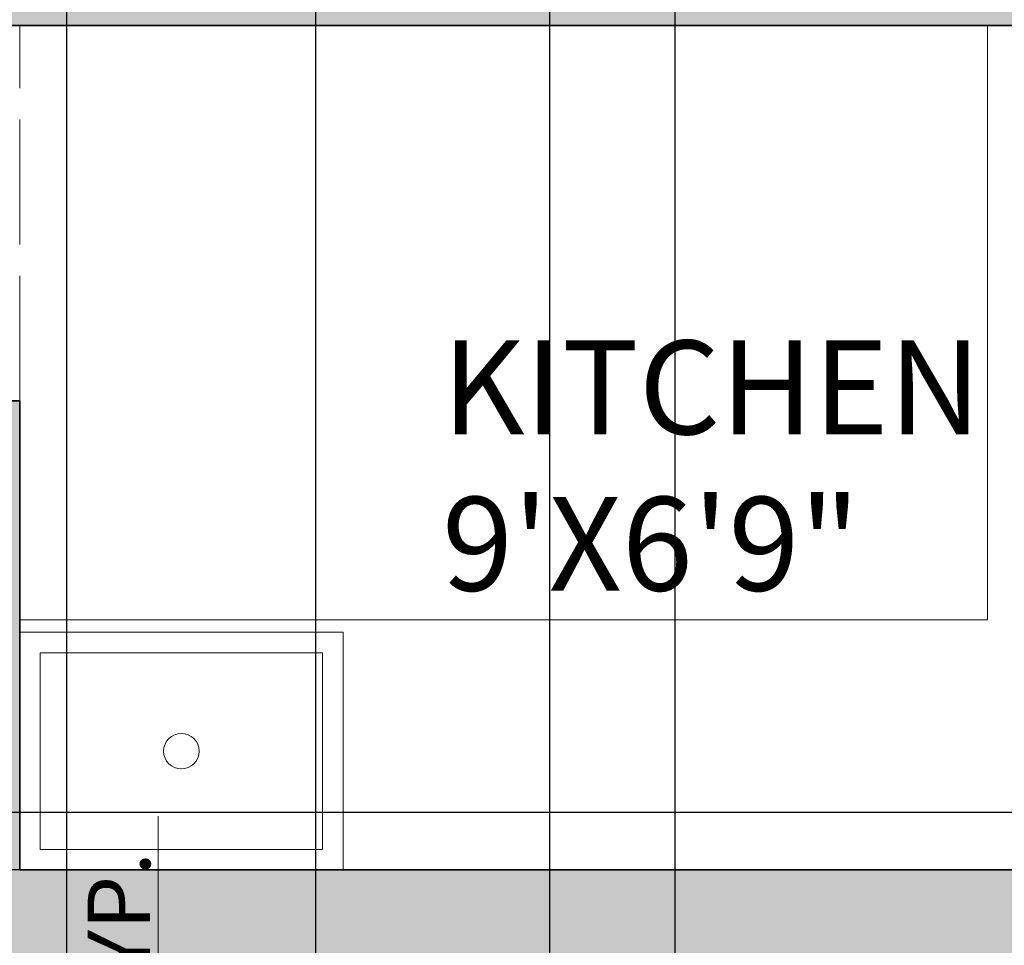
# Model space of a CAD drawing. Units: inches. Extents: x 2696 to 3240, y 1564 to 2310.
# Tile 65 of 76: x 3074 to 3168, y 1982 to 2071. Entities that reach past the tile are written whole.
import ezdxf

# ---------------------------------------------------------------- set-up
doc = ezdxf.new("R2010")
doc.units = ezdxf.units.IN
doc.linetypes.add('ACAD_ISO02W100', pattern=[15, 12, -3])
for name, color, linetype, lineweight in [('A-ANNO-DIMS', 3, 'Continuous', 18), ('A-AREA-IDEN', 7, 'Continuous', 18), ('A-FLOR-CASE', 8, 'Continuous', 18), ('A-FLOR-FIXT', 8, 'Continuous', 18), ('A-WALL', 7, 'Continuous', 35), ('A-WALL-OVHD', 7, 'ACAD_ISO02W100', 18), ('A-WALL-PATT', 9, 'Continuous', 13)]:
    doc.layers.add(name, color=color, linetype=linetype, lineweight=lineweight)
doc.styles.add('TIMES NEW', font='times.ttf')
doc.styles.add('YQ_DIM', font='SUPEROS.SHX', dxfattribs={"width": 0.8, "bigfont": 'HZDX.SHX'})
doc.dimstyles.new('Siddhuu', dxfattribs={"dimtxt": 6, "dimasz": 2.5, "dimexe": 1.25, "dimexo": 0.625, "dimtad": 1, "dimdec": 1, "dimlunit": 4, "dimtxsty": 'TIMES NEW', "dimcen": 2.5, "dimclrd": 256, "dimclre": 1, "dimclrt": 7, "dimadec": 0, "dimazin": 0, "dimtfac": 1, "dimtdec": 1, "dimtmove": 0, "dimatfit": 3, "dimfxl": 1, "dimtolj": 1, "dimlwd": -1, "dimarcsym": 0})

# ---------------------------------------------------------------- blocks, each defined once
blk = doc.blocks.new('SINK-KITCHEN')
for points in [[(0, 22.797), (31.038, 22.797), (31.038, 0), (0, 0)], [(1.972, 20.824), (29.066, 20.824), (29.066, 1.972), (1.972, 1.972)]]:
    blk.add_lwpolyline(points, close=True)
blk.add_circle((15.519, 11.398), 1.705)
blk = doc.blocks.new('*D48')
at = {"layer": 'A-ANNO-DIMS', "transparency": 16777216}
for p, q in [((3087, 1884.201), (3087, 1994.355)), ((3087, 1827.443), (3087, 1881.701))]:
    blk.add_line(p, q, dxfattribs=at)
at = {"layer": 'A-ANNO-DIMS', "color": 1, "lineweight": -2, "transparency": 16777216}
for p, q in [((3078.736, 1884.201), (3088.25, 1884.201)), ((3078.736, 1824.943), (3088.25, 1824.943))]:
    blk.add_line(p, q, dxfattribs=at)
at = {"layer": 'A-ANNO-DIMS', "transparency": 16777216}
for points in [[(3086.583, 1881.701), (3087.417, 1881.701), (3087, 1884.201)], [(3086.583, 1827.443), (3087.417, 1827.443), (3087, 1824.943)]]:
    blk.add_solid(points, dxfattribs=at)
at = {"layer": 'Defpoints', "color": 0, "transparency": 16777216}
for p in [(3078.111, 1884.201), (3087, 1884.201), (3078.111, 1824.943)]:
    blk.add_point(p, dxfattribs=at)
at = {"layer": 'A-ANNO-DIMS', "color": 7, "transparency": 16777216, "insert": (3083.232, 1940.528), "char_height": 6, "attachment_point": 5, "rotation": 90, "style": 'TIMES NEW'}
blk.add_mtext('\\A1;SECTIONAL 4\'-11 1/2" TYP.', dxfattribs=at)
blk = doc.blocks.new('*D54')
at = {"layer": 'A-ANNO-DIMS', "color": 1, "lineweight": -2, "transparency": 16777216}
for p, q in [((3124.611, 1893.826), (3124.611, 2298.451)), ((3136.611, 1893.826), (3136.611, 2298.451))]:
    blk.add_line(p, q, dxfattribs=at)
at = {"layer": 'A-ANNO-DIMS', "transparency": 16777216}
for p, q in [((3127.111, 2297.201), (3134.111, 2297.201)), ((3136.611, 2297.201), (3155.757, 2297.201))]:
    blk.add_line(p, q, dxfattribs=at)
for points in [[(3127.111, 2297.618), (3127.111, 2296.784), (3124.611, 2297.201)], [(3134.111, 2297.618), (3134.111, 2296.784), (3136.611, 2297.201)]]:
    blk.add_solid(points, dxfattribs=at)
at = {"layer": 'Defpoints', "color": 0, "transparency": 16777216}
for p in [(3136.611, 2297.201), (3124.611, 1893.201), (3136.611, 1893.201)]:
    blk.add_point(p, dxfattribs=at)
at = {"layer": 'A-ANNO-DIMS', "color": 7, "transparency": 16777216, "insert": (3147.434, 2300.878), "char_height": 6, "attachment_point": 5, "style": 'TIMES NEW'}
blk.add_mtext('\\A1;1\'-0"', dxfattribs=at)
blk = doc.blocks.new('*D65')
at = {"layer": 'A-ANNO-DIMS', "color": 1, "lineweight": -2, "transparency": 16777216}
for p, q in [((3078.209, 2122.076), (3078.209, 1568.951)), ((3102.111, 2122.076), (3102.111, 1568.951))]:
    blk.add_line(p, q, dxfattribs=at)
at = {"layer": 'A-ANNO-DIMS', "transparency": 16777216}
blk.add_line((3080.709, 1570.201), (3099.611, 1570.201), dxfattribs=at)
for points in [[(3080.709, 1570.618), (3080.709, 1569.784), (3078.209, 1570.201)], [(3099.611, 1570.618), (3099.611, 1569.784), (3102.111, 1570.201)]]:
    blk.add_solid(points, dxfattribs=at)
at = {"layer": 'Defpoints', "color": 0, "transparency": 16777216}
for p in [(3078.209, 2122.701), (3102.111, 2122.701), (3102.111, 1570.201)]:
    blk.add_point(p, dxfattribs=at)
at = {"layer": 'A-ANNO-DIMS', "color": 7, "transparency": 16777216, "insert": (3090.16, 1573.878), "char_height": 6, "attachment_point": 5, "style": 'TIMES NEW'}
blk.add_mtext('\\A1;2\'-0"', dxfattribs=at)
blk = doc.blocks.new('*D77')
at = {"layer": 'A-ANNO-DIMS', "transparency": 16777216}
for p, q in [((2710.611, 1997.201), (2710.611, 2030.601)), ((2710.611, 1989.201), (2710.611, 1994.701)), ((2710.611, 1986.701), (2710.611, 1984.201))]:
    blk.add_line(p, q, dxfattribs=at)
at = {"layer": 'A-ANNO-DIMS', "color": 1, "lineweight": -2, "transparency": 16777216}
for p, q in [((3189.986, 1994.701), (2709.361, 1994.701)), ((3189.986, 1989.201), (2709.361, 1989.201))]:
    blk.add_line(p, q, dxfattribs=at)
at = {"layer": 'A-ANNO-DIMS', "transparency": 16777216}
for points in [[(2710.195, 1997.201), (2711.028, 1997.201), (2710.611, 1994.701)], [(2710.195, 1986.701), (2711.028, 1986.701), (2710.611, 1989.201)]]:
    blk.add_solid(points, dxfattribs=at)
at = {"layer": 'Defpoints', "color": 0, "transparency": 16777216}
for p in [(2710.611, 1994.701), (3190.611, 1994.701), (3190.611, 1989.201)]:
    blk.add_point(p, dxfattribs=at)
at = {"layer": 'A-ANNO-DIMS', "color": 7, "transparency": 16777216, "insert": (2706.85, 2015.151), "char_height": 6, "attachment_point": 5, "rotation": 90, "style": 'TIMES NEW'}
blk.add_mtext('\\A1;0\'-5 1/2"', dxfattribs=at)

msp = doc.modelspace()

# ---------------------------------------------------------------- hatches: boundary and pattern name
at = {"layer": 'A-WALL-PATT', "transparency": 33554556}
h = msp.add_hatch(color=256, dxfattribs=at)
h.dxf.hatch_style = 1
h.paths.add_polyline_path([(2879.111, 2253.201), (2905.91, 2253.201), (2905.91, 2262.201), (2841.889, 2262.201), (2841.889, 2253.201), (2870.111, 2253.201), (2870.111, 2176.601), (2965.709, 2176.601), (2965.709, 2206.701), (2973.583, 2206.701), (2973.583, 2215.701), (2965.709, 2215.701), (2965.709, 2262.201), (2929.91, 2262.201), (2929.91, 2253.201), (2956.709, 2253.201), (2956.709, 2185.601), (2879.111, 2185.601)])
h.paths.add_polyline_path([(2782.834, 2262.201), (2745.611, 2262.201), (2745.611, 2228.729), (2754.611, 2228.729), (2754.611, 2253.201), (2782.834, 2253.201)])
h.paths.add_polyline_path([(2754.611, 2136.201), (2965.709, 2136.201), (2965.709, 2145.201), (2879.111, 2145.201), (2879.111, 2147.074), (2877.34, 2147.074), (2870.111, 2147.074), (2870.111, 2145.201), (2754.611, 2145.201), (2754.611, 2169.674), (2745.611, 2169.674), (2745.611, 2000.201), (2754.611, 2000.201), (2754.611, 2019.201), (2849.083, 2019.201), (2849.083, 2023.701), (2841.209, 2023.701), (2841.209, 2051.827), (2836.709, 2051.827), (2836.709, 2023.701), (2754.611, 2023.701), (2754.611, 2091.201), (2836.709, 2091.201), (2836.709, 2087.827), (2841.209, 2087.827), (2841.209, 2095.701), (2754.611, 2095.701)])
h.paths.add_polyline_path([(2965.709, 2136.201), (2956.709, 2136.201), (2956.709, 2023.701), (2885.083, 2023.701), (2885.083, 2019.201), (2956.709, 2019.201), (2956.709, 1950.575), (2965.709, 1950.575), (2965.709, 1980.201), (2973.583, 1980.201), (2973.583, 1989.201), (2965.709, 1989.201)])
h.paths.add_polyline_path([(2754.611, 1906.701), (2880.209, 1906.701), (2884.709, 1906.701), (2956.709, 1906.701), (2956.709, 1792.701), (2944.709, 1792.701), (2944.709, 1783.701), (2956.709, 1783.701), (2956.709, 1740.201), (2884.709, 1740.201), (2884.709, 1783.701), (2896.709, 1783.701), (2896.709, 1792.701), (2884.709, 1792.701), (2884.709, 1846.701), (2880.209, 1846.701), (2880.209, 1740.201), (2754.611, 1740.201), (2754.611, 1777.201), (2745.611, 1777.201), (2745.611, 1692.701), (2754.611, 1692.701), (2754.611, 1731.201), (2956.709, 1731.201), (2956.709, 1723.327), (2965.709, 1723.327), (2965.709, 1884.201), (2973.583, 1884.201), (2973.583, 1893.201), (2965.709, 1893.201), (2965.709, 1914.575), (2956.709, 1914.575), (2956.709, 1911.201), (2754.611, 1911.201), (2754.611, 1930.201), (2745.611, 1930.201), (2745.611, 1817.201), (2754.611, 1817.201), (2754.611, 1854.201), (2826.611, 1854.201), (2826.611, 1868.827), (2822.111, 1868.827), (2822.111, 1858.701), (2754.611, 1858.701)])
h.paths.add_polyline_path([(2965.709, 1656.201), (3008.237, 1656.201), (3008.237, 1665.201), (2965.709, 1665.201), (2965.709, 1693.327), (2956.709, 1693.327), (2956.709, 1686.201), (2934.583, 1686.201), (2934.583, 1681.701), (2956.709, 1681.701), (2956.709, 1614.201), (2896.709, 1614.201), (2896.709, 1681.701), (2904.583, 1681.701), (2904.583, 1686.201), (2892.209, 1686.201), (2892.209, 1614.201), (2858.41, 1614.201), (2858.41, 1605.201), (2965.709, 1605.201)])
h.paths.add_polyline_path([(2788.41, 1614.201), (2754.611, 1614.201), (2754.611, 1652.701), (2745.611, 1652.701), (2745.611, 1605.201), (2788.41, 1605.201)])
h.paths.add_polyline_path([(3199.611, 1633.048), (3190.611, 1633.048), (3190.611, 1614.201), (3082.611, 1614.201), (3082.611, 1665.201), (3070.237, 1665.201), (3070.237, 1656.201), (3078.111, 1656.201), (3078.111, 1605.201), (3199.611, 1605.201)])
h.paths.add_polyline_path([(3199.611, 1702.048), (3190.611, 1702.048), (3190.611, 1699.701), (3106.611, 1699.701), (3106.611, 1747.701), (3190.611, 1747.701), (3190.611, 1752.201), (3082.611, 1752.201), (3082.611, 1760.075), (3078.111, 1760.075), (3078.111, 1747.701), (3102.111, 1747.701), (3102.111, 1699.701), (3078.111, 1699.701), (3078.111, 1695.201), (3190.611, 1695.201), (3190.611, 1676.355), (3199.611, 1676.355)])
h.paths.add_polyline_path([(3199.611, 1783.201), (3190.611, 1783.201), (3190.611, 1745.355), (3199.611, 1745.355)])
h.paths.add_polyline_path([(3082.611, 1884.201), (3190.611, 1884.201), (3190.611, 1853.201), (3199.611, 1853.201), (3199.611, 1901.701), (3190.611, 1901.701), (3190.611, 1893.201), (3005.583, 1893.201), (3005.583, 1891.281), (3005.583, 1884.201), (3078.111, 1884.201), (3078.111, 1792.075), (3082.611, 1792.075)])
h.paths.add_polyline_path([(3199.611, 1994.701), (3190.611, 1994.701), (3190.611, 1989.201), (3073.709, 1989.201), (3073.709, 2034.201), (3069.209, 2034.201), (3069.209, 1989.201), (3005.583, 1989.201), (3005.583, 1980.201), (3190.611, 1980.201), (3190.611, 1971.701), (3199.611, 1971.701)])
h.paths.add_polyline_path([(3199.611, 2155.201), (3190.611, 2155.201), (3190.611, 2064.701), (3199.611, 2064.701)])
h.paths.add_polyline_path([(3190.611, 2074.701), (3106.611, 2074.701), (3106.611, 2122.701), (3190.611, 2122.701), (3190.611, 2127.201), (3082.709, 2127.201), (3082.709, 2135.075), (3073.709, 2135.075), (3073.709, 2122.701), (3102.111, 2122.701), (3102.111, 2074.701), (3069.209, 2074.701), (3069.209, 2070.201), (3190.611, 2070.201)])
h.paths.add_polyline_path([(3082.709, 2253.201), (3190.611, 2253.201), (3190.611, 2225.201), (3199.611, 2225.201), (3199.611, 2262.201), (3073.709, 2262.201), (3073.709, 2215.701), (3035.583, 2215.701), (3035.583, 2206.701), (3073.709, 2206.701), (3073.709, 2171.075), (3082.709, 2171.075)])

# ---------------------------------------------------------------- linework, layer by layer
at = {"layer": 'A-FLOR-CASE'}
for p, q in [((3166.611, 2013.201), (3166.611, 2070.201)), ((3073.709, 2013.201), (3166.611, 2013.201))]:
    msp.add_line(p, q, dxfattribs=at)
at = {"layer": 'A-WALL'}
for p, q in [((3069.209, 2070.201), (3190.611, 2070.201)), ((3069.209, 2034.201), (3073.709, 2034.201)), ((3073.709, 2034.201), (3073.709, 1989.201)), ((3073.709, 1989.201), (3190.611, 1989.201))]:
    msp.add_line(p, q, dxfattribs=at)
at = {"layer": 'A-WALL-OVHD'}
msp.add_line((3073.709, 2034.201), (3073.709, 2070.201), dxfattribs=at)

# ---------------------------------------------------------------- block references
at = {"layer": 'A-FLOR-FIXT'}
msp.add_blockref('SINK-KITCHEN', (3073.709, 1989.201), dxfattribs=at)

# ---------------------------------------------------------------- texts
at = {"layer": 'A-AREA-IDEN', "insert": (3114.246, 2039.99), "char_height": 9, "attachment_point": 1, "style": 'YQ_DIM'}
msp.add_mtext_dynamic_manual_height_columns('KITCHEN\\P9\'X6\'9"', width=48.00324, gutter_width=12.5, heights=[0], dxfattribs=at)

# ---------------------------------------------------------------- dimensions: what is measured, and where the dimension line sits
at = {"layer": 'A-ANNO-DIMS'}
for base, p1, p2, picture, middle in [((3136.611, 2297.201), (3124.611, 1893.201), (3136.611, 1893.201), '*D54', (3147.434, 2300.878)), ((3102.111, 1570.201), (3078.209, 2122.701), (3102.111, 2122.701), '*D65', (3090.16, 1573.878))]:
    dim = msp.add_linear_dim(base=base, p1=p1, p2=p2, dimstyle='Siddhuu', override={"dimdec": 1, "dimlfac": 1, "dimrnd": 0, "dimzin": 1, "dimdsep": 46, "dimlunit": 4, "dimfrac": 2}, dxfattribs=at)
    dim.commit()
    dim.dimension.update_dxf_attribs({"geometry": picture, "text_midpoint": middle})
dim = msp.add_linear_dim(base=(2710.611, 1994.701), p1=(3190.611, 1989.201), p2=(3190.611, 1994.701), angle=90, dimstyle='Siddhuu', override={"dimdec": 1, "dimlfac": 1, "dimrnd": 0, "dimzin": 1, "dimdsep": 46, "dimlunit": 4, "dimfrac": 2}, dxfattribs=at)
dim.commit()
dim.dimension.update_dxf_attribs({"geometry": '*D77', "text_midpoint": (2706.85, 2015.151)})
dim = msp.add_linear_dim(base=(3087, 1884.201), p1=(3078.111, 1824.943), p2=(3078.111, 1884.201), angle=90, text='SECTIONAL <> TYP.', dimstyle='Siddhuu', override={"dimdec": 1, "dimlfac": 1, "dimrnd": 0, "dimzin": 1, "dimdsep": 46, "dimlunit": 4, "dimfrac": 2}, dxfattribs=at)
dim.commit()
dim.dimension.update_dxf_attribs({"geometry": '*D48', "text_midpoint": (3083.232, 1940.528)})

doc.saveas('drawing.dxf')
